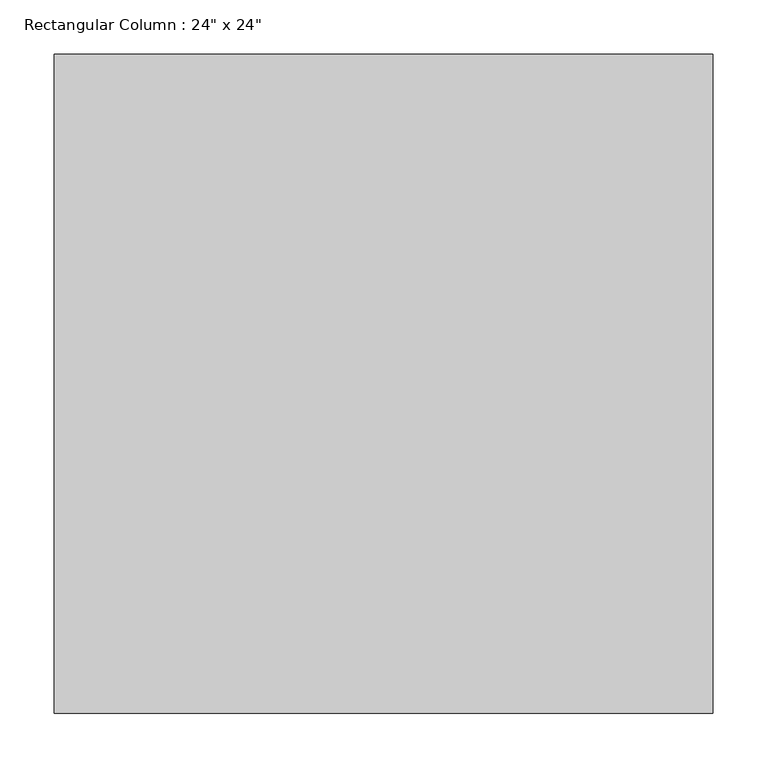
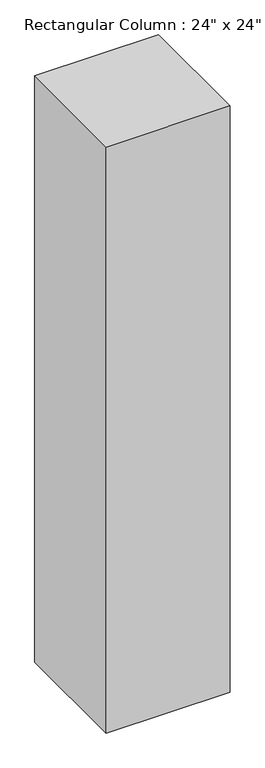
"""IFC4 building model written with IfcOpenShell, lengths in millimetres: column geometry."""

from ifc_helpers import new_model, si_unit, frame, origin, place, context, project, spatial, polyline, outline, extrude, source, transform, mapped, element, save


def column_8afb6978(model_context):
    return source(origin(), model_context, "Body", "SweptSolid", [
        extrude(outline(polyline([(304.8, 304.8), (304.8, -304.8), (-304.8, -304.8), (-304.8, 304.8), (304.8, 304.8)])), frame((0.0, 0.0, 3200.4), z_axis=(0.0, 0.0, 1.0), x_axis=(1.0, 0.0, 0.0)), (0.0, 0.0, 1.0), 3048.0),
    ])


if __name__ == "__main__":
    model = new_model("IFC4")
    model_context = context("Model", 3, world=origin())
    ifc_project = project(units=[si_unit("LENGTHUNIT", "METRE", prefix="MILLI")], contexts=[model_context])
    site = spatial("IfcSite", under=ifc_project)
    building = spatial("IfcBuilding", under=site)
    placement = place(None, origin())
    column_shape = column_8afb6978(model_context)
    element("IfcColumn", 1, ObjectType="Rectangular Column : 24\" x 24\"", at=placement, inside=building, context=model_context, shape_type="MappedRepresentation", body=[
        mapped(column_shape, transform((0.0, 0.0, 0.0), x_axis=(1.0, 0.0, 0.0), y_axis=(0.0, 1.0, 0.0), z_axis=(0.0, 0.0, 1.0))),
    ])
    save(model, "model.ifc")

# Revit data of these elements
# Type "Rectangular Column : 24\" x 24\""
#   Assembly Code = "B1010200"
#   Depth = 2' - 0"
#   Offset Base = 0' - 0"
#   Offset Top = 0' - 0"
#   Width = 2' - 0"
#   Material = none
